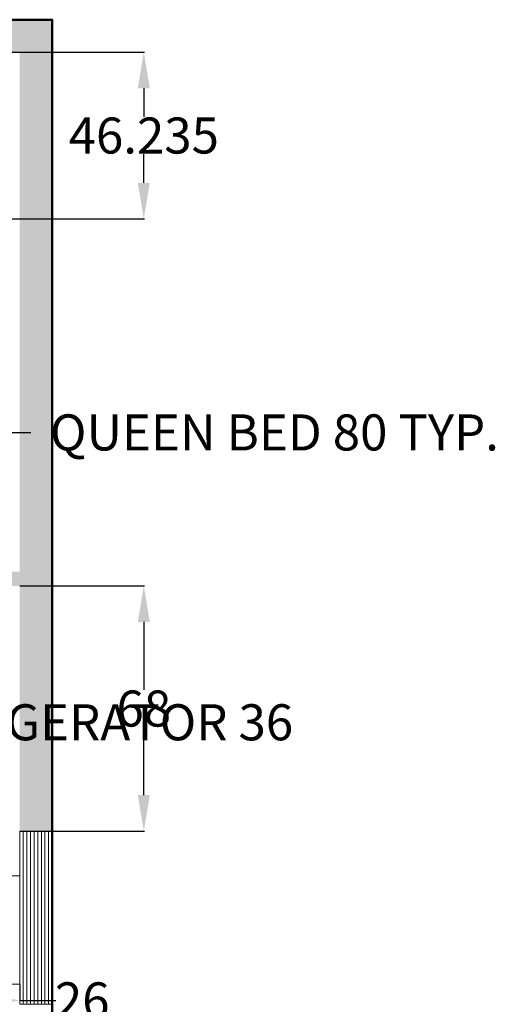
# Model space of a CAD drawing. Units: inches. Extents: x 133 to 758, y -29 to 543.
# Tile 7 of 7: x 626 to 758, y 235 to 508. Entities that reach past the tile are written whole.
import ezdxf

# ---------------------------------------------------------------- set-up
doc = ezdxf.new("R2010")
doc.units = ezdxf.units.IN
doc.header["$MEASUREMENT"] = 0
for name, color, linetype, lineweight in [('A-ANNO-DIMS', 2, 'Continuous', 18), ('A-EQPM', 8, 'Continuous', 20), ('A-WALL', 7, 'Continuous', 50), ('WINDOW', 151, 'Continuous', 18)]:
    doc.layers.add(name, color=color, linetype=linetype, lineweight=lineweight)
doc.layers.add('A-WALL-PATT', color=251, linetype='Continuous', lineweight=13, true_color=0x636466)
doc.styles.get("Standard").update_dxf_attribs({"font": 'arial.ttf'})
doc.dimstyles.get("Standard").update_dxf_attribs({"dimtxt": 10, "dimasz": 10, "dimexe": 0.18, "dimexo": 0.0625, "dimgap": 0.09, "dimtad": 0, "dimtih": 1, "dimtoh": 1, "dimdec": 0, "dimzin": 0, "dimdsep": 46, "dimlunit": 4, "dimtxsty": 'Standard', "dimcen": 0.09, "dimadec": 0, "dimazin": 0, "dimtfac": 1, "dimtdec": 0, "dimtofl": 0, "dimtmove": 0, "dimatfit": 3, "dimfxl": 1, "dimtolj": 1, "dimtzin": 0, "dimarcsym": 0})

# ---------------------------------------------------------------- blocks, each defined once
blk = doc.blocks.new('Range-Oven - 30 in top')
for p, q in [((0, -3), (30, -3)), ((12, -6), (18, -6)), ((13, -20), (13, -6)), ((14, -6), (14, -20)), ((15, -20), (15, -6)), ((16, -6), (16, -20)), ((17, -20), (17, -6)), ((18, -20), (12, -20)), ((6, -24), (6, -25)), ((8, -25), (8, -24)), ((22, -25), (22, -24)), ((24, -24), (24, -25))]:
    blk.add_line(p, q)
for points in [[(0, -24), (0, 0), (30, 0), (30, -24)], [(12, -21), (12, -5), (18, -5), (18, -21)], [(2, -26), (2, -25), (28, -25), (28, -26)]]:
    blk.add_lwpolyline(points, close=True)
for centre, radius in [((6, -9), 4), ((6, -9), 3), ((6, -9), 2), ((6, -9), 1), ((24, -9), 3), ((24, -9), 2), ((24, -9), 1), ((6, -18), 3), ((6, -18), 2), ((24, -18), 4), ((24, -18), 3), ((24, -18), 2), ((6, -18), 1), ((24, -18), 1)]:
    blk.add_circle(centre, radius)
blk = doc.blocks.new('WIN-48IN')
for p, q in [((0, 8), (48, 8)), ((0, 7), (48, 7)), ((0, 6), (48, 6)), ((0, 5), (48, 5)), ((0, 4), (48, 4)), ((0, 3), (48, 3)), ((0, 2), (48, 2)), ((0, 1), (48, 1)), ((0, 0), (48, 0))]:
    blk.add_line(p, q)
blk.add_lwpolyline([(48, 9), (48, 0), (0, 0), (0, 9)], close=True)
blk = doc.blocks.new('*D44')
at = {"layer": 'A-ANNO-DIMS', "color": 0, "lineweight": -2, "transparency": 16777216}
for p, q in [((538.86, 405.84), (538.86, 393.72)), ((618.86, 405.84), (618.86, 393.72)), ((548.86, 393.9), (608.86, 393.9)), ((618.86, 393.9), (628.86, 393.9))]:
    blk.add_line(p, q, dxfattribs=at)
at = {"layer": 'A-ANNO-DIMS', "color": 0, "transparency": 16777216}
for points in [[(548.86, 395.56), (548.86, 392.23), (538.86, 393.9)], [(608.86, 395.56), (608.86, 392.23), (618.86, 393.9)]]:
    blk.add_solid(points, dxfattribs=at)
at = {"layer": 'Defpoints', "color": 0, "transparency": 16777216}
for p in [(538.86, 405.9), (618.86, 405.9), (618.86, 393.9)]:
    blk.add_point(p, dxfattribs=at)
at = {"layer": 'A-ANNO-DIMS', "color": 0, "transparency": 16777216, "insert": (696.36, 393.9), "char_height": 10, "attachment_point": 5}
blk.add_mtext('\\A1;QUEEN BED 80 TYP.', dxfattribs=at)
blk = doc.blocks.new('*D63')
at = {"layer": 'A-ANNO-DIMS', "color": 0, "lineweight": -2, "transparency": 16777216}
for p, q in [((599.75, 240.86), (599.75, 236.24)), ((625.75, 240.86), (625.75, 236.24)), ((609.75, 236.42), (615.75, 236.42)), ((625.75, 236.42), (635.75, 236.42))]:
    blk.add_line(p, q, dxfattribs=at)
at = {"layer": 'A-ANNO-DIMS', "color": 0, "transparency": 16777216}
for points in [[(609.75, 238.09), (609.75, 234.75), (599.75, 236.42)], [(615.75, 238.09), (615.75, 234.75), (625.75, 236.42)]]:
    blk.add_solid(points, dxfattribs=at)
at = {"layer": 'Defpoints', "color": 0, "transparency": 16777216}
for p in [(599.75, 240.92), (625.75, 240.92), (625.75, 236.42)]:
    blk.add_point(p, dxfattribs=at)
at = {"layer": 'A-ANNO-DIMS', "color": 0, "transparency": 16777216, "insert": (643.08, 236.42), "char_height": 10, "attachment_point": 5}
blk.add_mtext('\\A1;26', dxfattribs=at)
blk = doc.blocks.new('*D66')
at = {"layer": 'A-ANNO-DIMS', "color": 0, "lineweight": -2, "transparency": 16777216}
for p, q in [((532.9, 318.87), (532.9, 313.35)), ((568.9, 318.87), (568.9, 313.35)), ((542.9, 313.53), (558.9, 313.53)), ((568.9, 313.53), (578.9, 313.53))]:
    blk.add_line(p, q, dxfattribs=at)
at = {"layer": 'A-ANNO-DIMS', "color": 0, "transparency": 16777216}
for points in [[(542.9, 315.2), (542.9, 311.86), (532.9, 313.53)], [(558.9, 315.2), (558.9, 311.86), (568.9, 313.53)]]:
    blk.add_solid(points, dxfattribs=at)
at = {"layer": 'Defpoints', "color": 0, "transparency": 16777216}
for p in [(532.9, 318.93), (568.9, 318.93), (568.9, 313.53)]:
    blk.add_point(p, dxfattribs=at)
at = {"layer": 'A-ANNO-DIMS', "color": 0, "transparency": 16777216, "insert": (643.33, 313.53), "char_height": 10, "attachment_point": 5}
blk.add_mtext('\\A1;REFRIGERATOR 36', dxfattribs=at)
blk = doc.blocks.new('*D82')
at = {"layer": 'A-ANNO-DIMS', "color": 0, "lineweight": -2, "transparency": 16777216}
for p, q in [((625.81, 351.34), (660.33, 351.34)), ((660.15, 341.34), (660.15, 322.53)), ((660.15, 293.34), (660.15, 312.14)), ((625.81, 283.34), (660.33, 283.34))]:
    blk.add_line(p, q, dxfattribs=at)
at = {"layer": 'A-ANNO-DIMS', "color": 0, "transparency": 16777216}
for points in [[(658.48, 341.34), (661.82, 341.34), (660.15, 351.34)], [(658.48, 293.34), (661.82, 293.34), (660.15, 283.34)]]:
    blk.add_solid(points, dxfattribs=at)
at = {"layer": 'Defpoints', "color": 0, "transparency": 16777216}
for p in [(625.75, 351.34), (625.75, 283.34), (660.15, 283.34)]:
    blk.add_point(p, dxfattribs=at)
at = {"layer": 'A-ANNO-DIMS', "color": 0, "transparency": 16777216, "insert": (660.15, 317.34), "char_height": 10, "attachment_point": 5}
blk.add_mtext('\\A1;68', dxfattribs=at)
blk = doc.blocks.new('*D98')
at = {"layer": 'A-ANNO-DIMS', "color": 0, "lineweight": -2, "transparency": 16777216}
for p, q in [((491.81, 499.34), (660.33, 499.34)), ((660.15, 489.34), (660.15, 481.42)), ((660.15, 463.1), (660.15, 471.02)), ((489.4, 453.1), (660.33, 453.1))]:
    blk.add_line(p, q, dxfattribs=at)
at = {"layer": 'A-ANNO-DIMS', "color": 0, "transparency": 16777216}
for points in [[(658.48, 489.34), (661.82, 489.34), (660.15, 499.34)], [(658.48, 463.1), (661.82, 463.1), (660.15, 453.1)]]:
    blk.add_solid(points, dxfattribs=at)
at = {"layer": 'Defpoints', "color": 0, "transparency": 16777216}
for p in [(491.75, 499.34), (660.15, 499.34), (489.34, 453.1)]:
    blk.add_point(p, dxfattribs=at)
at = {"layer": 'A-ANNO-DIMS', "color": 0, "transparency": 16777216, "insert": (660.15, 476.22), "char_height": 10, "attachment_point": 5}
blk.add_mtext('\\A1;46.235', dxfattribs=at)

msp = doc.modelspace()

# ---------------------------------------------------------------- hatches: boundary and pattern name
at = {"layer": 'A-WALL-PATT'}
h = msp.add_hatch(color=256, dxfattribs=at)
h.dxf.hatch_style = 1
h.paths.add_polyline_path([(433.7501, 508.336), (349.7501, 508.336), (349.7501, 499.336), (385.7501, 499.336), (385.7501, 403.336), (385.7501, 355.336), (379.7501, 355.336), (379.7501, 351.336), (389.7501, 351.336), (389.7501, 399.336), (415.7501, 399.336), (415.7501, 403.336), (389.7501, 403.336), (389.7501, 499.336), (433.7501, 499.336)])
h.paths.add_polyline_path([(541.7501, 508.336), (457.7501, 508.336), (457.7501, 499.336), (491.7501, 499.336), (491.7501, 403.336), (445.7501, 403.336), (445.7501, 399.336), (491.7501, 399.336), (491.7501, 351.336), (495.7501, 351.336), (495.7501, 399.336), (495.7501, 499.336), (513.7501, 499.336), (541.7501, 499.336)])
h.paths.add_polyline_path([(634.7501, 508.336), (589.7501, 508.336), (589.7501, 499.336), (625.7501, 499.336), (625.7501, 355.336), (525.7501, 355.336), (525.7501, 351.336), (525.7501, 307.336), (529.7501, 307.336), (529.7501, 351.336), (625.7501, 351.336), (625.7501, 283.336), (634.7501, 283.336)])
h.paths.add_polyline_path([(301.7501, 508.336), (256.7501, 508.336), (256.7501, 283.336), (265.7501, 283.336), (265.7501, 351.336), (349.7501, 351.336), (349.7501, 355.336), (265.7501, 355.336), (265.7501, 499.336), (301.7501, 499.336)])
h.paths.add_polyline_path([(361.7501, 167.336), (265.7501, 167.336), (265.7501, 235.336), (256.7501, 235.336), (256.7501, 10.336), (309.4362, 10.336), (309.4362, 19.336), (265.7501, 19.336), (265.7501, 163.336), (283.7501, 163.336), (361.7501, 163.336)])

# ---------------------------------------------------------------- linework, layer by layer
at = {"layer": 'A-WALL'}
msp.add_lwpolyline([(505.7501, 10.336), (256.7501, 10.336), (256.7501, 508.336), (634.7501, 508.336), (634.7501, 10.336), (601.3503, 10.336)], dxfattribs=at)

# ---------------------------------------------------------------- block references
at = {"layer": 'A-EQPM', "rotation": 270}
msp.add_blockref('Range-Oven - 30 in top', (625.7501, 270.9203), dxfattribs=at)
at = {"layer": 'WINDOW', "rotation": 270.0000000000001}
msp.add_blockref('WIN-48IN', (625.7501, 283.3362), dxfattribs=at)

# ---------------------------------------------------------------- dimensions: what is measured, and where the dimension line sits
at = {"layer": 'A-ANNO-DIMS'}
for base, p1, p2, override, picture, middle in [((660.1501, 499.336), (489.3397, 453.1011), (491.7501, 499.336), {"dimdec": 3, "dimlfac": 1, "dimrnd": 0, "dimzin": 0, "dimdsep": 46, "dimlunit": 2}, '*D98', (660.1501, 476.2186)), ((660.1501, 283.336), (625.7501, 351.336), (625.7501, 283.336), {"dimdec": 0, "dimlfac": 1, "dimrnd": 0, "dimzin": 0, "dimdsep": 46, "dimlunit": 2}, '*D82', (660.1501, 317.336))]:
    dim = msp.add_linear_dim(base=base, p1=p1, p2=p2, angle=90, dimstyle='Standard', override=override, dxfattribs=at)
    dim.commit()
    dim.dimension.update_dxf_attribs({"geometry": picture, "text_midpoint": middle})
for base, p1, p2, text, picture, middle in [((618.8575, 393.8976), (538.8574, 405.8976), (618.8575, 405.8976), 'QUEEN BED <> TYP.', '*D44', (696.3588, 393.8976)), ((568.9033, 313.5301), (532.9033, 318.9301), (568.9033, 318.9301), 'REFRIGERATOR <>', '*D66', (643.3282, 313.5301))]:
    dim = msp.add_linear_dim(base=base, p1=p1, p2=p2, text=text, dimstyle='Standard', override={"dimdec": 0, "dimlfac": 1, "dimrnd": 0, "dimzin": 0, "dimdsep": 46, "dimlunit": 2}, dxfattribs=at)
    dim.commit()
    dim.dimension.update_dxf_attribs({"geometry": picture, "text_midpoint": middle})
dim = msp.add_linear_dim(base=(625.7501, 236.4203), p1=(599.7501, 240.9203), p2=(625.7501, 240.9203), dimstyle='Standard', override={"dimdec": 0, "dimlfac": 1, "dimrnd": 0, "dimzin": 0, "dimdsep": 46, "dimlunit": 2}, dxfattribs=at)
dim.commit()
dim.dimension.update_dxf_attribs({"geometry": '*D63', "text_midpoint": (643.0843, 236.4203)})

doc.saveas('drawing.dxf')
